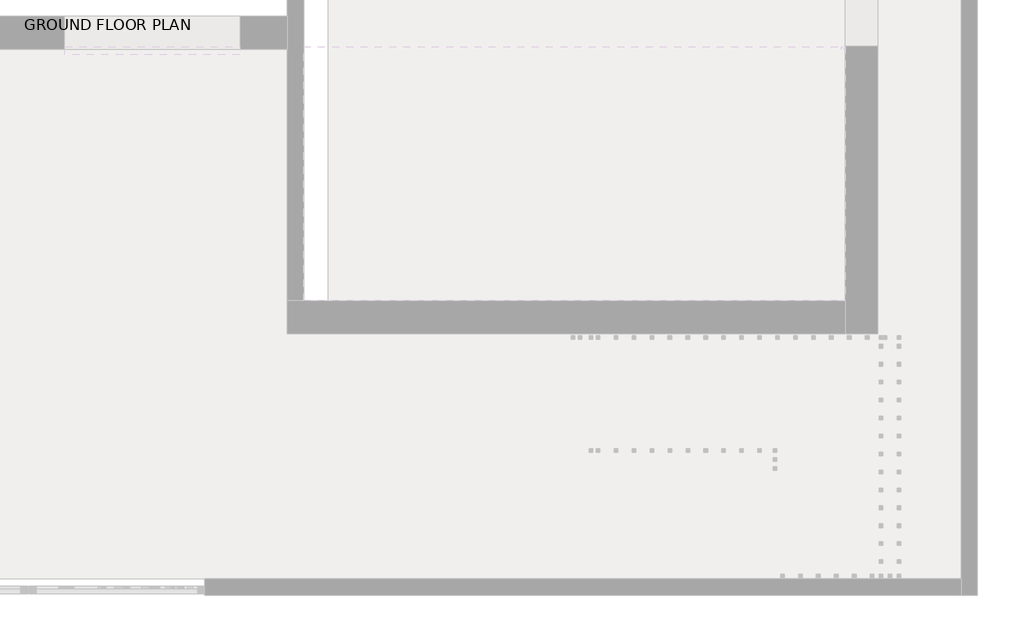
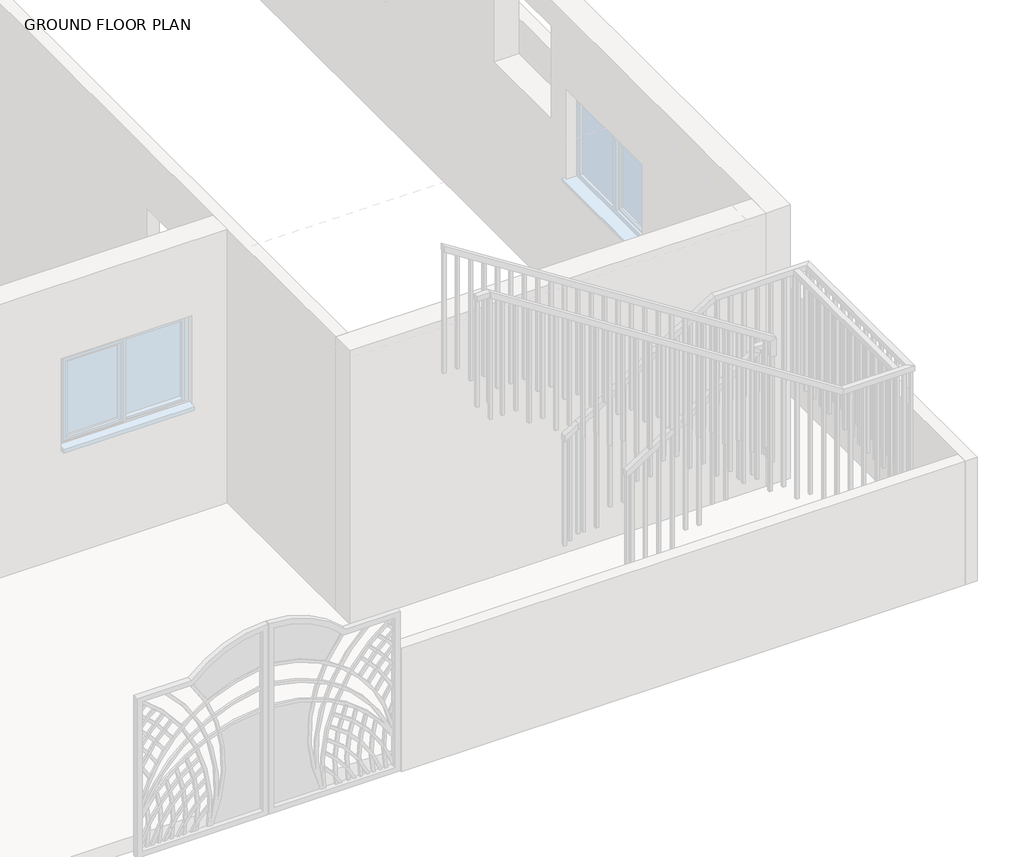
# One storey, part 3 of 23: 2 railings.
"""IFC4 building model written with IfcOpenShell, lengths in millimetres."""

from ifc_helpers import new_model, si_unit, frame, origin, place, context, project, spatial, polyline, outline, extrude, faceted_brep, element, save

model = new_model("IFC4")

# Units and contexts
model_context = context("Model", 3, world=origin())
ifc_project = project(units=[si_unit("LENGTHUNIT", "METRE", prefix="MILLI")], contexts=[model_context])

# Site, building, storey
site = spatial("IfcSite", under=ifc_project)
building = spatial("IfcBuilding", under=site)
storey = spatial("IfcBuildingStorey", under=building, Name="GROUND FLOOR PLAN", Elevation=487.68)

# Railings
placement = place(None, origin())
element("IfcRailing", 1, ObjectType="1100mm", at=placement, inside=storey, context=model_context, shape_type="SolidModel", body=[
    faceted_brep([(-8680.149573, -11007.9255223, 1912.8), (-8680.149573, -11007.9255223, 1853.4423995), (-8680.149573, -11057.9255223, 1853.4423995), (-8680.149573, -11057.9255223, 1912.8), (-7484.3306254, -11007.9255223, 2677.8717446), (-7434.3306254, -11007.9255223, 2650.5035914), (-7434.3306254, -11057.9255223, 2650.5035914), (-7484.3306254, -11057.9255223, 2677.8717446), (-7484.3306254, -11007.9255223, 2725.6), (-7434.3306254, -11007.9255223, 2675.6), (-7434.3306254, -11057.9255223, 2675.6), (-7484.3306254, -11057.9255223, 2725.6), (-7359.3306254, -11007.9255223, 2725.6), (-7359.3306254, -11007.9255223, 2675.6), (-7409.3306254, -11057.9255223, 2675.6), (-7409.3306254, -11057.9255223, 2725.6), (-7359.3306254, -11132.9255223, 2725.6), (-7359.3306254, -11132.9255223, 2675.6), (-7409.3306254, -11132.9255223, 2675.6), (-7409.3306254, -11132.9255223, 2725.6), (-7359.3306254, -11134.9255223, 2725.6), (-7409.3306254, -11134.9255223, 2725.6), (-7409.3306254, -11184.9255223, 2675.6), (-7359.3306254, -11184.9255223, 2675.6)], [[[0, 1, 2, 3]], [[1, 0, 4, 5]], [[2, 1, 5, 6]], [[3, 2, 6, 7]], [[0, 3, 7, 4]], [[5, 4, 8, 9]], [[6, 5, 9, 10]], [[7, 6, 10, 11]], [[4, 7, 11, 8]], [[9, 8, 12, 13]], [[10, 9, 13, 14]], [[11, 10, 14, 15]], [[8, 11, 15, 12]], [[13, 12, 16, 17]], [[14, 13, 17, 18]], [[15, 14, 18, 19]], [[12, 15, 19, 16]], [[20, 21, 22, 23]], [[17, 16, 20, 23]], [[18, 17, 23, 22]], [[19, 18, 22, 21]], [[16, 19, 21, 20]]]),
    faceted_brep([(-7359.3306254, -11134.9255223, 2725.6), (-7359.3306254, -11184.9255223, 2675.6), (-7409.3306254, -11184.9255223, 2675.6), (-7409.3306254, -11134.9255223, 2725.6), (-7359.3306254, -11134.9255223, 2855.9055527), (-7409.3306254, -11134.9255223, 2828.5415543), (-7409.3306254, -11184.9255223, 2828.5415543), (-7359.3306254, -11184.9255223, 2855.9055527)], [[[0, 1, 2, 3]], [[4, 5, 6, 7]], [[1, 0, 4, 7]], [[2, 1, 7, 6]], [[3, 2, 6, 5]], [[0, 3, 5, 4]]]),
    faceted_brep([(-7359.3306254, -11184.9255223, 2855.9055527), (-7409.3306254, -11184.9255223, 2828.5415543), (-7409.3306254, -11134.9255223, 2828.5415543), (-7359.3306254, -11134.9255223, 2855.9055527), (-10457.8773536, -11184.9255223, 4838.88), (-10457.8773536, -11134.9255223, 4838.88), (-10457.8773536, -11134.9255223, 4779.517542), (-10457.8773536, -11184.9255223, 4779.517542)], [[[0, 1, 2, 3]], [[4, 5, 6, 7]], [[1, 0, 4, 7]], [[2, 1, 7, 6]], [[3, 2, 6, 5]], [[0, 3, 5, 4]]]),
    extrude(outline(polyline([(3576.32, -10434.3306254), (4764.4483614, -10434.3306254), (4780.4475912, -10459.3306254), (3576.32, -10459.3306254), (3576.32, -10434.3306254)])), frame((0.0, -11172.4255223, 0.0), z_axis=(0.0, 1.0, 0.0), x_axis=(0.0, 0.0, 1.0)), (0.0, 0.0, 1.0), 25.0),
    extrude(outline(polyline([(3576.32, -10309.3306254), (4684.4522123, -10309.3306254), (4700.4514422, -10334.3306254), (3576.32, -10334.3306254), (3576.32, -10309.3306254)])), frame((0.0, -11172.4255223, 0.0), z_axis=(0.0, 1.0, 0.0), x_axis=(0.0, 0.0, 1.0)), (0.0, 0.0, 1.0), 25.0),
    extrude(outline(polyline([(3413.76, -10184.3306254), (4604.4560633, -10184.3306254), (4620.4552931, -10209.3306254), (3413.76, -10209.3306254), (3413.76, -10184.3306254)])), frame((0.0, -11172.4255223, 0.0), z_axis=(0.0, 1.0, 0.0), x_axis=(0.0, 0.0, 1.0)), (0.0, 0.0, 1.0), 25.0),
    extrude(outline(polyline([(3413.76, -10059.3306254), (4524.4599142, -10059.3306254), (4540.459144, -10084.3306254), (3413.76, -10084.3306254), (3413.76, -10059.3306254)])), frame((0.0, -11172.4255223, 0.0), z_axis=(0.0, 1.0, 0.0), x_axis=(0.0, 0.0, 1.0)), (0.0, 0.0, 1.0), 25.0),
    extrude(outline(polyline([(3251.2, -9934.3306254), (4444.4637652, -9934.3306254), (4460.462995, -9959.3306254), (3251.2, -9959.3306254), (3251.2, -9934.3306254)])), frame((0.0, -11172.4255223, 0.0), z_axis=(0.0, 1.0, 0.0), x_axis=(0.0, 0.0, 1.0)), (0.0, 0.0, 1.0), 25.0),
    extrude(outline(polyline([(3251.2, -9809.3306254), (4364.4676161, -9809.3306254), (4380.4668459, -9834.3306254), (3251.2, -9834.3306254), (3251.2, -9809.3306254)])), frame((0.0, -11172.4255223, 0.0), z_axis=(0.0, 1.0, 0.0), x_axis=(0.0, 0.0, 1.0)), (0.0, 0.0, 1.0), 25.0),
    extrude(outline(polyline([(3251.2, -9684.3306254), (4284.4714671, -9684.3306254), (4300.4706969, -9709.3306254), (3251.2, -9709.3306254), (3251.2, -9684.3306254)])), frame((0.0, -11172.4255223, 0.0), z_axis=(0.0, 1.0, 0.0), x_axis=(0.0, 0.0, 1.0)), (0.0, 0.0, 1.0), 25.0),
    extrude(outline(polyline([(3088.64, -9559.3306254), (4204.475318, -9559.3306254), (4220.4745478, -9584.3306254), (3088.64, -9584.3306254), (3088.64, -9559.3306254)])), frame((0.0, -11172.4255223, 0.0), z_axis=(0.0, 1.0, 0.0), x_axis=(0.0, 0.0, 1.0)), (0.0, 0.0, 1.0), 25.0),
    extrude(outline(polyline([(3088.64, -9434.3306254), (4124.479169, -9434.3306254), (4140.4783988, -9459.3306254), (3088.64, -9459.3306254), (3088.64, -9434.3306254)])), frame((0.0, -11172.4255223, 0.0), z_axis=(0.0, 1.0, 0.0), x_axis=(0.0, 0.0, 1.0)), (0.0, 0.0, 1.0), 25.0),
    extrude(outline(polyline([(2926.08, -9309.3306254), (4044.4830199, -9309.3306254), (4060.4822497, -9334.3306254), (2926.08, -9334.3306254), (2926.08, -9309.3306254)])), frame((0.0, -11172.4255223, 0.0), z_axis=(0.0, 1.0, 0.0), x_axis=(0.0, 0.0, 1.0)), (0.0, 0.0, 1.0), 25.0),
    extrude(outline(polyline([(2926.08, -9184.3306254), (3964.4868709, -9184.3306254), (3980.4861007, -9209.3306254), (2926.08, -9209.3306254), (2926.08, -9184.3306254)])), frame((0.0, -11172.4255223, 0.0), z_axis=(0.0, 1.0, 0.0), x_axis=(0.0, 0.0, 1.0)), (0.0, 0.0, 1.0), 25.0),
    extrude(outline(polyline([(2763.52, -9059.3306254), (3884.4907218, -9059.3306254), (3900.4899516, -9084.3306254), (2763.52, -9084.3306254), (2763.52, -9059.3306254)])), frame((0.0, -11172.4255223, 0.0), z_axis=(0.0, 1.0, 0.0), x_axis=(0.0, 0.0, 1.0)), (0.0, 0.0, 1.0), 25.0),
    extrude(outline(polyline([(2763.52, -8934.3306254), (3804.4945728, -8934.3306254), (3820.4938026, -8959.3306254), (2763.52, -8959.3306254), (2763.52, -8934.3306254)])), frame((0.0, -11172.4255223, 0.0), z_axis=(0.0, 1.0, 0.0), x_axis=(0.0, 0.0, 1.0)), (0.0, 0.0, 1.0), 25.0),
    extrude(outline(polyline([(2600.96, -8809.3306254), (3724.4984237, -8809.3306254), (3740.4976535, -8834.3306254), (2600.96, -8834.3306254), (2600.96, -8809.3306254)])), frame((0.0, -11172.4255223, 0.0), z_axis=(0.0, 1.0, 0.0), x_axis=(0.0, 0.0, 1.0)), (0.0, 0.0, 1.0), 25.0),
    extrude(outline(polyline([(2600.96, -8684.3306254), (3644.5022747, -8684.3306254), (3660.5015045, -8709.3306254), (2600.96, -8709.3306254), (2600.96, -8684.3306254)])), frame((0.0, -11172.4255223, 0.0), z_axis=(0.0, 1.0, 0.0), x_axis=(0.0, 0.0, 1.0)), (0.0, 0.0, 1.0), 25.0),
    extrude(outline(polyline([(2438.4, -8559.3306254), (3564.5061256, -8559.3306254), (3580.5053554, -8584.3306254), (2438.4, -8584.3306254), (2438.4, -8559.3306254)])), frame((0.0, -11172.4255223, 0.0), z_axis=(0.0, 1.0, 0.0), x_axis=(0.0, 0.0, 1.0)), (0.0, 0.0, 1.0), 25.0),
    extrude(outline(polyline([(2438.4, -8434.3306254), (3484.5099766, -8434.3306254), (3500.5092064, -8459.3306254), (2438.4, -8459.3306254), (2438.4, -8434.3306254)])), frame((0.0, -11172.4255223, 0.0), z_axis=(0.0, 1.0, 0.0), x_axis=(0.0, 0.0, 1.0)), (0.0, 0.0, 1.0), 25.0),
    extrude(outline(polyline([(2275.84, -8309.3306254), (3404.5138275, -8309.3306254), (3420.5130573, -8334.3306254), (2275.84, -8334.3306254), (2275.84, -8309.3306254)])), frame((0.0, -11172.4255223, 0.0), z_axis=(0.0, 1.0, 0.0), x_axis=(0.0, 0.0, 1.0)), (0.0, 0.0, 1.0), 25.0),
    extrude(outline(polyline([(2275.84, -8184.3306254), (3324.5176785, -8184.3306254), (3340.5169083, -8209.3306254), (2275.84, -8209.3306254), (2275.84, -8184.3306254)])), frame((0.0, -11172.4255223, 0.0), z_axis=(0.0, 1.0, 0.0), x_axis=(0.0, 0.0, 1.0)), (0.0, 0.0, 1.0), 25.0),
    extrude(outline(polyline([(2113.28, -8059.3306254), (3244.5215294, -8059.3306254), (3260.5207592, -8084.3306254), (2113.28, -8084.3306254), (2113.28, -8059.3306254)])), frame((0.0, -11172.4255223, 0.0), z_axis=(0.0, 1.0, 0.0), x_axis=(0.0, 0.0, 1.0)), (0.0, 0.0, 1.0), 25.0),
    extrude(outline(polyline([(2113.28, -7934.3306254), (3164.5253804, -7934.3306254), (3180.5246102, -7959.3306254), (2113.28, -7959.3306254), (2113.28, -7934.3306254)])), frame((0.0, -11172.4255223, 0.0), z_axis=(0.0, 1.0, 0.0), x_axis=(0.0, 0.0, 1.0)), (0.0, 0.0, 1.0), 25.0),
    extrude(outline(polyline([(1950.72, -7809.3306254), (3084.5292313, -7809.3306254), (3100.5284611, -7834.3306254), (1950.72, -7834.3306254), (1950.72, -7809.3306254)])), frame((0.0, -11172.4255223, 0.0), z_axis=(0.0, 1.0, 0.0), x_axis=(0.0, 0.0, 1.0)), (0.0, 0.0, 1.0), 25.0),
    extrude(outline(polyline([(1950.72, -7684.3306254), (3004.5330823, -7684.3306254), (3020.5323121, -7709.3306254), (1950.72, -7709.3306254), (1950.72, -7684.3306254)])), frame((0.0, -11172.4255223, 0.0), z_axis=(0.0, 1.0, 0.0), x_axis=(0.0, 0.0, 1.0)), (0.0, 0.0, 1.0), 25.0),
    extrude(outline(polyline([(1788.16, -7559.3306254), (2924.5369332, -7559.3306254), (2940.536163, -7584.3306254), (1788.16, -7584.3306254), (1788.16, -7559.3306254)])), frame((0.0, -11172.4255223, 0.0), z_axis=(0.0, 1.0, 0.0), x_axis=(0.0, 0.0, 1.0)), (0.0, 0.0, 1.0), 25.0),
    extrude(outline(polyline([(1788.16, -7434.3306254), (2844.5407841, -7434.3306254), (2860.540014, -7459.3306254), (1788.16, -7459.3306254), (1788.16, -7434.3306254)])), frame((0.0, -11172.4255223, 0.0), z_axis=(0.0, 1.0, 0.0), x_axis=(0.0, 0.0, 1.0)), (0.0, 0.0, 1.0), 25.0),
    extrude(outline(polyline([(-7396.8306254, -11082.9255223), (-7371.8306254, -11082.9255223), (-7371.8306254, -11107.9255223), (-7396.8306254, -11107.9255223), (-7396.8306254, -11082.9255223)])), frame((0.0, 0.0, 1625.6), z_axis=(0.0, 0.0, 1.0), x_axis=(1.0, 0.0, 0.0)), (0.0, 0.0, 1.0), 1050.0),
    extrude(outline(polyline([(2605.1944115, -7505.149573), (1463.04, -7505.149573), (1463.04, -7480.149573), (2621.1891352, -7480.149573), (2605.1944115, -7505.149573)])), frame((0.0, -11045.4255223, 0.0), z_axis=(0.0, 1.0, 0.0), x_axis=(0.0, 0.0, 1.0)), (0.0, 0.0, 1.0), 25.0),
    extrude(outline(polyline([(2525.2207932, -7630.149573), (1463.04, -7630.149573), (1463.04, -7605.149573), (2541.2155169, -7605.149573), (2525.2207932, -7630.149573)])), frame((0.0, -11045.4255223, 0.0), z_axis=(0.0, 1.0, 0.0), x_axis=(0.0, 0.0, 1.0)), (0.0, 0.0, 1.0), 25.0),
    extrude(outline(polyline([(2445.2471749, -7755.149573), (1300.48, -7755.149573), (1300.48, -7730.149573), (2461.2418986, -7730.149573), (2445.2471749, -7755.149573)])), frame((0.0, -11045.4255223, 0.0), z_axis=(0.0, 1.0, 0.0), x_axis=(0.0, 0.0, 1.0)), (0.0, 0.0, 1.0), 25.0),
    extrude(outline(polyline([(2365.2735566, -7880.149573), (1300.48, -7880.149573), (1300.48, -7855.149573), (2381.2682803, -7855.149573), (2365.2735566, -7880.149573)])), frame((0.0, -11045.4255223, 0.0), z_axis=(0.0, 1.0, 0.0), x_axis=(0.0, 0.0, 1.0)), (0.0, 0.0, 1.0), 25.0),
    extrude(outline(polyline([(2285.2999383, -8005.149573), (1137.92, -8005.149573), (1137.92, -7980.149573), (2301.294662, -7980.149573), (2285.2999383, -8005.149573)])), frame((0.0, -11045.4255223, 0.0), z_axis=(0.0, 1.0, 0.0), x_axis=(0.0, 0.0, 1.0)), (0.0, 0.0, 1.0), 25.0),
    extrude(outline(polyline([(2205.32632, -8130.149573), (1137.92, -8130.149573), (1137.92, -8105.149573), (2221.3210437, -8105.149573), (2205.32632, -8130.149573)])), frame((0.0, -11045.4255223, 0.0), z_axis=(0.0, 1.0, 0.0), x_axis=(0.0, 0.0, 1.0)), (0.0, 0.0, 1.0), 25.0),
    extrude(outline(polyline([(2125.3527017, -8255.149573), (975.36, -8255.149573), (975.36, -8230.149573), (2141.3474254, -8230.149573), (2125.3527017, -8255.149573)])), frame((0.0, -11045.4255223, 0.0), z_axis=(0.0, 1.0, 0.0), x_axis=(0.0, 0.0, 1.0)), (0.0, 0.0, 1.0), 25.0),
    extrude(outline(polyline([(2045.3790834, -8380.149573), (975.36, -8380.149573), (975.36, -8355.149573), (2061.3738071, -8355.149573), (2045.3790834, -8380.149573)])), frame((0.0, -11045.4255223, 0.0), z_axis=(0.0, 1.0, 0.0), x_axis=(0.0, 0.0, 1.0)), (0.0, 0.0, 1.0), 25.0),
    extrude(outline(polyline([(1965.4054651, -8505.149573), (812.8, -8505.149573), (812.8, -8480.149573), (1981.4001888, -8480.149573), (1965.4054651, -8505.149573)])), frame((0.0, -11045.4255223, 0.0), z_axis=(0.0, 1.0, 0.0), x_axis=(0.0, 0.0, 1.0)), (0.0, 0.0, 1.0), 25.0),
    extrude(outline(polyline([(1885.4318468, -8630.149573), (812.8, -8630.149573), (812.8, -8605.149573), (1901.4265705, -8605.149573), (1885.4318468, -8630.149573)])), frame((0.0, -11045.4255223, 0.0), z_axis=(0.0, 1.0, 0.0), x_axis=(0.0, 0.0, 1.0)), (0.0, 0.0, 1.0), 25.0),
    extrude(outline(polyline([(-7396.8306254, -11147.4255223), (-7371.8306254, -11147.4255223), (-7371.8306254, -11172.4255223), (-7396.8306254, -11172.4255223), (-7396.8306254, -11147.4255223)])), frame((0.0, 0.0, 1625.6), z_axis=(0.0, 0.0, 1.0), x_axis=(1.0, 0.0, 0.0)), (0.0, 0.0, 1.0), 1050.0),
    extrude(outline(polyline([(-7396.8306254, -11045.4255223), (-7396.8306254, -11020.4255223), (-7371.8306254, -11020.4255223), (-7371.8306254, -11045.4255223), (-7396.8306254, -11045.4255223)])), frame((0.0, 0.0, 1625.6), z_axis=(0.0, 0.0, 1.0), x_axis=(1.0, 0.0, 0.0)), (0.0, 0.0, 1.0), 1050.0),
    extrude(outline(polyline([(3576.32, -10432.8773536), (4763.5183122, -10432.8773536), (4779.517542, -10457.8773536), (3576.32, -10457.8773536), (3576.32, -10432.8773536)])), frame((0.0, -11172.4255223, 0.0), z_axis=(0.0, 1.0, 0.0), x_axis=(0.0, 0.0, 1.0)), (0.0, 0.0, 1.0), 25.0),
    extrude(outline(polyline([(1853.4423995, -8680.149573), (812.8, -8680.149573), (812.8, -8655.149573), (1869.4371231, -8655.149573), (1853.4423995, -8680.149573)])), frame((0.0, -11045.4255223, 0.0), z_axis=(0.0, 1.0, 0.0), x_axis=(0.0, 0.0, 1.0)), (0.0, 0.0, 1.0), 25.0),
])
element("IfcRailing", 2, ObjectType="1100mm", at=placement, inside=storey, context=model_context, shape_type="SolidModel", body=[
    faceted_brep([(-8680.149573, -10220.0521308, 1912.8), (-8680.149573, -10220.0521308, 1853.4423995), (-8680.149573, -10270.0521308, 1853.4423995), (-8680.149573, -10270.0521308, 1912.8), (-7409.7306254, -10220.0521308, 2725.6), (-7395.1045513, -10220.0521308, 2675.6), (-7395.1045513, -10270.0521308, 2675.6), (-7409.7306254, -10270.0521308, 2725.6), (-6495.8132565, -10220.0521308, 2725.6), (-6495.8132565, -10220.0521308, 2675.6), (-6545.8132565, -10270.0521308, 2675.6), (-6545.8132565, -10270.0521308, 2725.6), (-6495.8132565, -11933.6860066, 2725.6), (-6495.8132565, -11933.6860066, 2675.6), (-6545.8132565, -11883.6860066, 2675.6), (-6545.8132565, -11883.6860066, 2725.6), (-7155.718398, -11933.6860066, 2725.6), (-7170.3479429, -11933.6860066, 2675.6), (-7170.3479429, -11883.6860066, 2675.6), (-7155.718398, -11883.6860066, 2725.6), (-10457.8773536, -11933.6860066, 4838.88), (-10457.8773536, -11883.6860066, 4838.88), (-10457.8773536, -11883.6860066, 4779.517542), (-10457.8773536, -11933.6860066, 4779.517542)], [[[0, 1, 2, 3]], [[1, 0, 4, 5]], [[2, 1, 5, 6]], [[3, 2, 6, 7]], [[0, 3, 7, 4]], [[5, 4, 8, 9]], [[6, 5, 9, 10]], [[7, 6, 10, 11]], [[4, 7, 11, 8]], [[9, 8, 12, 13]], [[10, 9, 13, 14]], [[11, 10, 14, 15]], [[8, 11, 15, 12]], [[13, 12, 16, 17]], [[14, 13, 17, 18]], [[15, 14, 18, 19]], [[12, 15, 19, 16]], [[20, 21, 22, 23]], [[17, 16, 20, 23]], [[18, 17, 23, 22]], [[19, 18, 22, 21]], [[16, 19, 21, 20]]]),
    extrude(outline(polyline([(4691.8007425, -10320.8132565), (4707.7999723, -10345.8132565), (3576.32, -10345.8132565), (3576.32, -10320.8132565), (4691.8007425, -10320.8132565)])), frame((0.0, -11921.1860066, 0.0), z_axis=(0.0, 1.0, 0.0), x_axis=(0.0, 0.0, 1.0)), (0.0, 0.0, 1.0), 25.0),
    extrude(outline(polyline([(4611.8045935, -10195.8132565), (4627.8038233, -10220.8132565), (3576.32, -10220.8132565), (3576.32, -10195.8132565), (4611.8045935, -10195.8132565)])), frame((0.0, -11921.1860066, 0.0), z_axis=(0.0, 1.0, 0.0), x_axis=(0.0, 0.0, 1.0)), (0.0, 0.0, 1.0), 25.0),
    extrude(outline(polyline([(4531.8084444, -10070.8132565), (4547.8076742, -10095.8132565), (3413.76, -10095.8132565), (3413.76, -10070.8132565), (4531.8084444, -10070.8132565)])), frame((0.0, -11921.1860066, 0.0), z_axis=(0.0, 1.0, 0.0), x_axis=(0.0, 0.0, 1.0)), (0.0, 0.0, 1.0), 25.0),
    extrude(outline(polyline([(4451.8122954, -9945.8132565), (4467.8115252, -9970.8132565), (3413.76, -9970.8132565), (3413.76, -9945.8132565), (4451.8122954, -9945.8132565)])), frame((0.0, -11921.1860066, 0.0), z_axis=(0.0, 1.0, 0.0), x_axis=(0.0, 0.0, 1.0)), (0.0, 0.0, 1.0), 25.0),
    extrude(outline(polyline([(4371.8161463, -9820.8132565), (4387.8153761, -9845.8132565), (3251.2, -9845.8132565), (3251.2, -9820.8132565), (4371.8161463, -9820.8132565)])), frame((0.0, -11921.1860066, 0.0), z_axis=(0.0, 1.0, 0.0), x_axis=(0.0, 0.0, 1.0)), (0.0, 0.0, 1.0), 25.0),
    extrude(outline(polyline([(4291.8423995, -9695.8132565), (4307.8371231, -9720.8132565), (3251.2, -9720.8132565), (3251.2, -9695.8132565), (4291.8423995, -9695.8132565)])), frame((0.0, -11921.1860066, 0.0), z_axis=(0.0, 1.0, 0.0), x_axis=(0.0, 0.0, 1.0)), (0.0, 0.0, 1.0), 25.0),
    extrude(outline(polyline([(4211.8238482, -9570.8132565), (4227.823078, -9595.8132565), (3088.64, -9595.8132565), (3088.64, -9570.8132565), (4211.8238482, -9570.8132565)])), frame((0.0, -11921.1860066, 0.0), z_axis=(0.0, 1.0, 0.0), x_axis=(0.0, 0.0, 1.0)), (0.0, 0.0, 1.0), 25.0),
    extrude(outline(polyline([(4131.8276992, -9445.8132565), (4147.826929, -9470.8132565), (3088.64, -9470.8132565), (3088.64, -9445.8132565), (4131.8276992, -9445.8132565)])), frame((0.0, -11921.1860066, 0.0), z_axis=(0.0, 1.0, 0.0), x_axis=(0.0, 0.0, 1.0)), (0.0, 0.0, 1.0), 25.0),
    extrude(outline(polyline([(4051.8315501, -9320.8132565), (4067.8307799, -9345.8132565), (2926.08, -9345.8132565), (2926.08, -9320.8132565), (4051.8315501, -9320.8132565)])), frame((0.0, -11921.1860066, 0.0), z_axis=(0.0, 1.0, 0.0), x_axis=(0.0, 0.0, 1.0)), (0.0, 0.0, 1.0), 25.0),
    extrude(outline(polyline([(3971.835401, -9195.8132565), (3987.8346309, -9220.8132565), (2926.08, -9220.8132565), (2926.08, -9195.8132565), (3971.835401, -9195.8132565)])), frame((0.0, -11921.1860066, 0.0), z_axis=(0.0, 1.0, 0.0), x_axis=(0.0, 0.0, 1.0)), (0.0, 0.0, 1.0), 25.0),
    extrude(outline(polyline([(3891.839252, -9070.8132565), (3907.8384818, -9095.8132565), (2763.52, -9095.8132565), (2763.52, -9070.8132565), (3891.839252, -9070.8132565)])), frame((0.0, -11921.1860066, 0.0), z_axis=(0.0, 1.0, 0.0), x_axis=(0.0, 0.0, 1.0)), (0.0, 0.0, 1.0), 25.0),
    extrude(outline(polyline([(3811.8431029, -8945.8132565), (3827.8423328, -8970.8132565), (2763.52, -8970.8132565), (2763.52, -8945.8132565), (3811.8431029, -8945.8132565)])), frame((0.0, -11921.1860066, 0.0), z_axis=(0.0, 1.0, 0.0), x_axis=(0.0, 0.0, 1.0)), (0.0, 0.0, 1.0), 25.0),
    extrude(outline(polyline([(3731.8469539, -8820.8132565), (3747.8461837, -8845.8132565), (2600.96, -8845.8132565), (2600.96, -8820.8132565), (3731.8469539, -8820.8132565)])), frame((0.0, -11921.1860066, 0.0), z_axis=(0.0, 1.0, 0.0), x_axis=(0.0, 0.0, 1.0)), (0.0, 0.0, 1.0), 25.0),
    extrude(outline(polyline([(3651.8508048, -8695.8132565), (3667.8500347, -8720.8132565), (2600.96, -8720.8132565), (2600.96, -8695.8132565), (3651.8508048, -8695.8132565)])), frame((0.0, -11921.1860066, 0.0), z_axis=(0.0, 1.0, 0.0), x_axis=(0.0, 0.0, 1.0)), (0.0, 0.0, 1.0), 25.0),
    extrude(outline(polyline([(3571.8546558, -8570.8132565), (3587.8538856, -8595.8132565), (2438.4, -8595.8132565), (2438.4, -8570.8132565), (3571.8546558, -8570.8132565)])), frame((0.0, -11921.1860066, 0.0), z_axis=(0.0, 1.0, 0.0), x_axis=(0.0, 0.0, 1.0)), (0.0, 0.0, 1.0), 25.0),
    extrude(outline(polyline([(3491.8585067, -8445.8132565), (3507.8577365, -8470.8132565), (2438.4, -8470.8132565), (2438.4, -8445.8132565), (3491.8585067, -8445.8132565)])), frame((0.0, -11921.1860066, 0.0), z_axis=(0.0, 1.0, 0.0), x_axis=(0.0, 0.0, 1.0)), (0.0, 0.0, 1.0), 25.0),
    extrude(outline(polyline([(3411.8623577, -8320.8132565), (3427.8615875, -8345.8132565), (2275.84, -8345.8132565), (2275.84, -8320.8132565), (3411.8623577, -8320.8132565)])), frame((0.0, -11921.1860066, 0.0), z_axis=(0.0, 1.0, 0.0), x_axis=(0.0, 0.0, 1.0)), (0.0, 0.0, 1.0), 25.0),
    extrude(outline(polyline([(3331.8662086, -8195.8132565), (3347.8654384, -8220.8132565), (2275.84, -8220.8132565), (2275.84, -8195.8132565), (3331.8662086, -8195.8132565)])), frame((0.0, -11921.1860066, 0.0), z_axis=(0.0, 1.0, 0.0), x_axis=(0.0, 0.0, 1.0)), (0.0, 0.0, 1.0), 25.0),
    extrude(outline(polyline([(3251.8700596, -8070.8132565), (3267.8692894, -8095.8132565), (2113.28, -8095.8132565), (2113.28, -8070.8132565), (3251.8700596, -8070.8132565)])), frame((0.0, -11921.1860066, 0.0), z_axis=(0.0, 1.0, 0.0), x_axis=(0.0, 0.0, 1.0)), (0.0, 0.0, 1.0), 25.0),
    extrude(outline(polyline([(3171.8739105, -7945.8132565), (3187.8731403, -7970.8132565), (2113.28, -7970.8132565), (2113.28, -7945.8132565), (3171.8739105, -7945.8132565)])), frame((0.0, -11921.1860066, 0.0), z_axis=(0.0, 1.0, 0.0), x_axis=(0.0, 0.0, 1.0)), (0.0, 0.0, 1.0), 25.0),
    extrude(outline(polyline([(3091.8777615, -7820.8132565), (3107.8769913, -7845.8132565), (1950.72, -7845.8132565), (1950.72, -7820.8132565), (3091.8777615, -7820.8132565)])), frame((0.0, -11921.1860066, 0.0), z_axis=(0.0, 1.0, 0.0), x_axis=(0.0, 0.0, 1.0)), (0.0, 0.0, 1.0), 25.0),
    extrude(outline(polyline([(3011.8816124, -7695.8132565), (3027.8808422, -7720.8132565), (1950.72, -7720.8132565), (1950.72, -7695.8132565), (3011.8816124, -7695.8132565)])), frame((0.0, -11921.1860066, 0.0), z_axis=(0.0, 1.0, 0.0), x_axis=(0.0, 0.0, 1.0)), (0.0, 0.0, 1.0), 25.0),
    extrude(outline(polyline([(2931.8854634, -7570.8132565), (2947.8846932, -7595.8132565), (1788.16, -7595.8132565), (1788.16, -7570.8132565), (2931.8854634, -7570.8132565)])), frame((0.0, -11921.1860066, 0.0), z_axis=(0.0, 1.0, 0.0), x_axis=(0.0, 0.0, 1.0)), (0.0, 0.0, 1.0), 25.0),
    extrude(outline(polyline([(2851.8893143, -7445.8132565), (2867.8885441, -7470.8132565), (1788.16, -7470.8132565), (1788.16, -7445.8132565), (2851.8893143, -7445.8132565)])), frame((0.0, -11921.1860066, 0.0), z_axis=(0.0, 1.0, 0.0), x_axis=(0.0, 0.0, 1.0)), (0.0, 0.0, 1.0), 25.0),
    extrude(outline(polyline([(2771.8931653, -7320.8132565), (2787.8923951, -7345.8132565), (1625.6, -7345.8132565), (1625.6, -7320.8132565), (2771.8931653, -7320.8132565)])), frame((0.0, -11921.1860066, 0.0), z_axis=(0.0, 1.0, 0.0), x_axis=(0.0, 0.0, 1.0)), (0.0, 0.0, 1.0), 25.0),
    extrude(outline(polyline([(2691.8970162, -7195.8132565), (2707.896246, -7220.8132565), (1625.6, -7220.8132565), (1625.6, -7195.8132565), (2691.8970162, -7195.8132565)])), frame((0.0, -11921.1860066, 0.0), z_axis=(0.0, 1.0, 0.0), x_axis=(0.0, 0.0, 1.0)), (0.0, 0.0, 1.0), 25.0),
    extrude(outline(polyline([(-7070.8132565, -11921.1860066), (-7095.8132565, -11921.1860066), (-7095.8132565, -11896.1860066), (-7070.8132565, -11896.1860066), (-7070.8132565, -11921.1860066)])), frame((0.0, 0.0, 1625.6), z_axis=(0.0, 0.0, 1.0), x_axis=(1.0, 0.0, 0.0)), (0.0, 0.0, 1.0), 1050.0),
    extrude(outline(polyline([(-6945.8132565, -11921.1860066), (-6970.8132565, -11921.1860066), (-6970.8132565, -11896.1860066), (-6945.8132565, -11896.1860066), (-6945.8132565, -11921.1860066)])), frame((0.0, 0.0, 1625.6), z_axis=(0.0, 0.0, 1.0), x_axis=(1.0, 0.0, 0.0)), (0.0, 0.0, 1.0), 1050.0),
    extrude(outline(polyline([(-6820.8132565, -11921.1860066), (-6845.8132565, -11921.1860066), (-6845.8132565, -11896.1860066), (-6820.8132565, -11896.1860066), (-6820.8132565, -11921.1860066)])), frame((0.0, 0.0, 1625.6), z_axis=(0.0, 0.0, 1.0), x_axis=(1.0, 0.0, 0.0)), (0.0, 0.0, 1.0), 1050.0),
    extrude(outline(polyline([(-6695.8132565, -11921.1860066), (-6720.8132565, -11921.1860066), (-6720.8132565, -11896.1860066), (-6695.8132565, -11896.1860066), (-6695.8132565, -11921.1860066)])), frame((0.0, 0.0, 1625.6), z_axis=(0.0, 0.0, 1.0), x_axis=(1.0, 0.0, 0.0)), (0.0, 0.0, 1.0), 1050.0),
    extrude(outline(polyline([(-6570.8132565, -11921.1860066), (-6595.8132565, -11921.1860066), (-6595.8132565, -11896.1860066), (-6570.8132565, -11896.1860066), (-6570.8132565, -11921.1860066)])), frame((0.0, 0.0, 1625.6), z_axis=(0.0, 0.0, 1.0), x_axis=(1.0, 0.0, 0.0)), (0.0, 0.0, 1.0), 1050.0),
    extrude(outline(polyline([(-6508.3132565, -11795.0521308), (-6508.3132565, -11820.0521308), (-6533.3132565, -11820.0521308), (-6533.3132565, -11795.0521308), (-6508.3132565, -11795.0521308)])), frame((0.0, 0.0, 1625.6), z_axis=(0.0, 0.0, 1.0), x_axis=(1.0, 0.0, 0.0)), (0.0, 0.0, 1.0), 1050.0),
    extrude(outline(polyline([(-6508.3132565, -11670.0521308), (-6508.3132565, -11695.0521308), (-6533.3132565, -11695.0521308), (-6533.3132565, -11670.0521308), (-6508.3132565, -11670.0521308)])), frame((0.0, 0.0, 1625.6), z_axis=(0.0, 0.0, 1.0), x_axis=(1.0, 0.0, 0.0)), (0.0, 0.0, 1.0), 1050.0),
    extrude(outline(polyline([(-6508.3132565, -11545.0521308), (-6508.3132565, -11570.0521308), (-6533.3132565, -11570.0521308), (-6533.3132565, -11545.0521308), (-6508.3132565, -11545.0521308)])), frame((0.0, 0.0, 1625.6), z_axis=(0.0, 0.0, 1.0), x_axis=(1.0, 0.0, 0.0)), (0.0, 0.0, 1.0), 1050.0),
    extrude(outline(polyline([(-6508.3132565, -11420.0521308), (-6508.3132565, -11445.0521308), (-6533.3132565, -11445.0521308), (-6533.3132565, -11420.0521308), (-6508.3132565, -11420.0521308)])), frame((0.0, 0.0, 1625.6), z_axis=(0.0, 0.0, 1.0), x_axis=(1.0, 0.0, 0.0)), (0.0, 0.0, 1.0), 1050.0),
    extrude(outline(polyline([(-6508.3132565, -11295.0521308), (-6508.3132565, -11320.0521308), (-6533.3132565, -11320.0521308), (-6533.3132565, -11295.0521308), (-6508.3132565, -11295.0521308)])), frame((0.0, 0.0, 1625.6), z_axis=(0.0, 0.0, 1.0), x_axis=(1.0, 0.0, 0.0)), (0.0, 0.0, 1.0), 1050.0),
    extrude(outline(polyline([(-6508.3132565, -11170.0521308), (-6508.3132565, -11195.0521308), (-6533.3132565, -11195.0521308), (-6533.3132565, -11170.0521308), (-6508.3132565, -11170.0521308)])), frame((0.0, 0.0, 1625.6), z_axis=(0.0, 0.0, 1.0), x_axis=(1.0, 0.0, 0.0)), (0.0, 0.0, 1.0), 1050.0),
    extrude(outline(polyline([(-6508.3132565, -11045.0521308), (-6508.3132565, -11070.0521308), (-6533.3132565, -11070.0521308), (-6533.3132565, -11045.0521308), (-6508.3132565, -11045.0521308)])), frame((0.0, 0.0, 1625.6), z_axis=(0.0, 0.0, 1.0), x_axis=(1.0, 0.0, 0.0)), (0.0, 0.0, 1.0), 1050.0),
    extrude(outline(polyline([(-6508.3132565, -10920.0521308), (-6508.3132565, -10945.0521308), (-6533.3132565, -10945.0521308), (-6533.3132565, -10920.0521308), (-6508.3132565, -10920.0521308)])), frame((0.0, 0.0, 1625.6), z_axis=(0.0, 0.0, 1.0), x_axis=(1.0, 0.0, 0.0)), (0.0, 0.0, 1.0), 1050.0),
    extrude(outline(polyline([(-6508.3132565, -10795.0521308), (-6508.3132565, -10820.0521308), (-6533.3132565, -10820.0521308), (-6533.3132565, -10795.0521308), (-6508.3132565, -10795.0521308)])), frame((0.0, 0.0, 1625.6), z_axis=(0.0, 0.0, 1.0), x_axis=(1.0, 0.0, 0.0)), (0.0, 0.0, 1.0), 1050.0),
    extrude(outline(polyline([(-6508.3132565, -10670.0521308), (-6508.3132565, -10695.0521308), (-6533.3132565, -10695.0521308), (-6533.3132565, -10670.0521308), (-6508.3132565, -10670.0521308)])), frame((0.0, 0.0, 1625.6), z_axis=(0.0, 0.0, 1.0), x_axis=(1.0, 0.0, 0.0)), (0.0, 0.0, 1.0), 1050.0),
    extrude(outline(polyline([(-6508.3132565, -10545.0521308), (-6508.3132565, -10570.0521308), (-6533.3132565, -10570.0521308), (-6533.3132565, -10545.0521308), (-6508.3132565, -10545.0521308)])), frame((0.0, 0.0, 1625.6), z_axis=(0.0, 0.0, 1.0), x_axis=(1.0, 0.0, 0.0)), (0.0, 0.0, 1.0), 1050.0),
    extrude(outline(polyline([(-6508.3132565, -10420.0521308), (-6508.3132565, -10445.0521308), (-6533.3132565, -10445.0521308), (-6533.3132565, -10420.0521308), (-6508.3132565, -10420.0521308)])), frame((0.0, 0.0, 1625.6), z_axis=(0.0, 0.0, 1.0), x_axis=(1.0, 0.0, 0.0)), (0.0, 0.0, 1.0), 1050.0),
    extrude(outline(polyline([(-6508.3132565, -10295.0521308), (-6508.3132565, -10320.0521308), (-6533.3132565, -10320.0521308), (-6533.3132565, -10295.0521308), (-6508.3132565, -10295.0521308)])), frame((0.0, 0.0, 1625.6), z_axis=(0.0, 0.0, 1.0), x_axis=(1.0, 0.0, 0.0)), (0.0, 0.0, 1.0), 1050.0),
    extrude(outline(polyline([(-6630.149573, -10232.5521308), (-6605.149573, -10232.5521308), (-6605.149573, -10257.5521308), (-6630.149573, -10257.5521308), (-6630.149573, -10232.5521308)])), frame((0.0, 0.0, 1625.6), z_axis=(0.0, 0.0, 1.0), x_axis=(1.0, 0.0, 0.0)), (0.0, 0.0, 1.0), 1050.0),
    extrude(outline(polyline([(-6755.149573, -10232.5521308), (-6730.149573, -10232.5521308), (-6730.149573, -10257.5521308), (-6755.149573, -10257.5521308), (-6755.149573, -10232.5521308)])), frame((0.0, 0.0, 1625.6), z_axis=(0.0, 0.0, 1.0), x_axis=(1.0, 0.0, 0.0)), (0.0, 0.0, 1.0), 1050.0),
    extrude(outline(polyline([(-6880.149573, -10232.5521308), (-6855.149573, -10232.5521308), (-6855.149573, -10257.5521308), (-6880.149573, -10257.5521308), (-6880.149573, -10232.5521308)])), frame((0.0, 0.0, 1625.6), z_axis=(0.0, 0.0, 1.0), x_axis=(1.0, 0.0, 0.0)), (0.0, 0.0, 1.0), 1050.0),
    extrude(outline(polyline([(-7005.149573, -10232.5521308), (-6980.149573, -10232.5521308), (-6980.149573, -10257.5521308), (-7005.149573, -10257.5521308), (-7005.149573, -10232.5521308)])), frame((0.0, 0.0, 1625.6), z_axis=(0.0, 0.0, 1.0), x_axis=(1.0, 0.0, 0.0)), (0.0, 0.0, 1.0), 1050.0),
    extrude(outline(polyline([(-7130.149573, -10232.5521308), (-7105.149573, -10232.5521308), (-7105.149573, -10257.5521308), (-7130.149573, -10257.5521308), (-7130.149573, -10232.5521308)])), frame((0.0, 0.0, 1625.6), z_axis=(0.0, 0.0, 1.0), x_axis=(1.0, 0.0, 0.0)), (0.0, 0.0, 1.0), 1050.0),
    extrude(outline(polyline([(-7255.149573, -10232.5521308), (-7230.149573, -10232.5521308), (-7230.149573, -10257.5521308), (-7255.149573, -10257.5521308), (-7255.149573, -10232.5521308)])), frame((0.0, 0.0, 1625.6), z_axis=(0.0, 0.0, 1.0), x_axis=(1.0, 0.0, 0.0)), (0.0, 0.0, 1.0), 1050.0),
    extrude(outline(polyline([(-7380.149573, -10232.5521308), (-7355.149573, -10232.5521308), (-7355.149573, -10257.5521308), (-7380.149573, -10257.5521308), (-7380.149573, -10232.5521308)])), frame((0.0, 0.0, 1625.6), z_axis=(0.0, 0.0, 1.0), x_axis=(1.0, 0.0, 0.0)), (0.0, 0.0, 1.0), 1050.0),
    extrude(outline(polyline([(1463.04, -7505.149573), (1463.04, -7480.149573), (2621.1891352, -7480.149573), (2605.1944115, -7505.149573), (1463.04, -7505.149573)])), frame((0.0, -10257.5521308, 0.0), z_axis=(0.0, 1.0, 0.0), x_axis=(0.0, 0.0, 1.0)), (0.0, 0.0, 1.0), 25.0),
    extrude(outline(polyline([(1463.04, -7630.149573), (1463.04, -7605.149573), (2541.2155169, -7605.149573), (2525.2207932, -7630.149573), (1463.04, -7630.149573)])), frame((0.0, -10257.5521308, 0.0), z_axis=(0.0, 1.0, 0.0), x_axis=(0.0, 0.0, 1.0)), (0.0, 0.0, 1.0), 25.0),
    extrude(outline(polyline([(1300.48, -7755.149573), (1300.48, -7730.149573), (2461.2418986, -7730.149573), (2445.2471749, -7755.149573), (1300.48, -7755.149573)])), frame((0.0, -10257.5521308, 0.0), z_axis=(0.0, 1.0, 0.0), x_axis=(0.0, 0.0, 1.0)), (0.0, 0.0, 1.0), 25.0),
    extrude(outline(polyline([(1300.48, -7880.149573), (1300.48, -7855.149573), (2381.2682803, -7855.149573), (2365.2735566, -7880.149573), (1300.48, -7880.149573)])), frame((0.0, -10257.5521308, 0.0), z_axis=(0.0, 1.0, 0.0), x_axis=(0.0, 0.0, 1.0)), (0.0, 0.0, 1.0), 25.0),
    extrude(outline(polyline([(1137.92, -8005.149573), (1137.92, -7980.149573), (2301.294662, -7980.149573), (2285.2999383, -8005.149573), (1137.92, -8005.149573)])), frame((0.0, -10257.5521308, 0.0), z_axis=(0.0, 1.0, 0.0), x_axis=(0.0, 0.0, 1.0)), (0.0, 0.0, 1.0), 25.0),
    extrude(outline(polyline([(1137.92, -8130.149573), (1137.92, -8105.149573), (2221.3210437, -8105.149573), (2205.32632, -8130.149573), (1137.92, -8130.149573)])), frame((0.0, -10257.5521308, 0.0), z_axis=(0.0, 1.0, 0.0), x_axis=(0.0, 0.0, 1.0)), (0.0, 0.0, 1.0), 25.0),
    extrude(outline(polyline([(975.36, -8255.149573), (975.36, -8230.149573), (2141.3474254, -8230.149573), (2125.3527017, -8255.149573), (975.36, -8255.149573)])), frame((0.0, -10257.5521308, 0.0), z_axis=(0.0, 1.0, 0.0), x_axis=(0.0, 0.0, 1.0)), (0.0, 0.0, 1.0), 25.0),
    extrude(outline(polyline([(975.36, -8380.149573), (975.36, -8355.149573), (2061.3738071, -8355.149573), (2045.3790834, -8380.149573), (975.36, -8380.149573)])), frame((0.0, -10257.5521308, 0.0), z_axis=(0.0, 1.0, 0.0), x_axis=(0.0, 0.0, 1.0)), (0.0, 0.0, 1.0), 25.0),
    extrude(outline(polyline([(812.8, -8505.149573), (812.8, -8480.149573), (1981.4001888, -8480.149573), (1965.4054651, -8505.149573), (812.8, -8505.149573)])), frame((0.0, -10257.5521308, 0.0), z_axis=(0.0, 1.0, 0.0), x_axis=(0.0, 0.0, 1.0)), (0.0, 0.0, 1.0), 25.0),
    extrude(outline(polyline([(812.8, -8630.149573), (812.8, -8605.149573), (1901.4265705, -8605.149573), (1885.4318468, -8630.149573), (812.8, -8630.149573)])), frame((0.0, -10257.5521308, 0.0), z_axis=(0.0, 1.0, 0.0), x_axis=(0.0, 0.0, 1.0)), (0.0, 0.0, 1.0), 25.0),
    extrude(outline(polyline([(-6508.3132565, -11896.1860066), (-6508.3132565, -11921.1860066), (-6533.3132565, -11921.1860066), (-6533.3132565, -11896.1860066), (-6508.3132565, -11896.1860066)])), frame((0.0, 0.0, 1625.6), z_axis=(0.0, 0.0, 1.0), x_axis=(1.0, 0.0, 0.0)), (0.0, 0.0, 1.0), 1050.0),
    extrude(outline(polyline([(-6533.3132565, -10232.5521308), (-6508.3132565, -10232.5521308), (-6508.3132565, -10257.5521308), (-6533.3132565, -10257.5521308), (-6533.3132565, -10232.5521308)])), frame((0.0, 0.0, 1625.6), z_axis=(0.0, 0.0, 1.0), x_axis=(1.0, 0.0, 0.0)), (0.0, 0.0, 1.0), 1050.0),
    extrude(outline(polyline([(4763.5183122, -10432.8773536), (4779.517542, -10457.8773536), (3576.32, -10457.8773536), (3576.32, -10432.8773536), (4763.5183122, -10432.8773536)])), frame((0.0, -11921.1860066, 0.0), z_axis=(0.0, 1.0, 0.0), x_axis=(0.0, 0.0, 1.0)), (0.0, 0.0, 1.0), 25.0),
    extrude(outline(polyline([(812.8, -8680.149573), (812.8, -8655.149573), (1869.4371231, -8655.149573), (1853.4423995, -8680.149573), (812.8, -8680.149573)])), frame((0.0, -10257.5521308, 0.0), z_axis=(0.0, 1.0, 0.0), x_axis=(0.0, 0.0, 1.0)), (0.0, 0.0, 1.0), 25.0),
])

save(model, "model.ifc")

# Revit data of these elements
# Type "1100mm"
#   built-in parameter 1008612 = 0.019685 (stored number, unit not read)
#   built-in parameter 1008611 = 0.019685 (stored number, unit not read)
#   built-in parameter 1008609 = 0.902231 (stored number, unit not read)
#   built-in parameter 1008604 = 0.19685 (stored number, unit not read)
#   built-in parameter 1008603 = 0.164042 (stored number, unit not read)
#   Railing Height = 3.608924 ft
#   built-in parameter 1008630 = 2
#   built-in parameter 1008610 = 2
#   built-in parameter 1008608 = 1
#   built-in parameter 1008618 = Baluster_Square : 25mm
# Elements 1, 2 (IfcRailing, "1100mm")
#   Phase Created = New Construction
